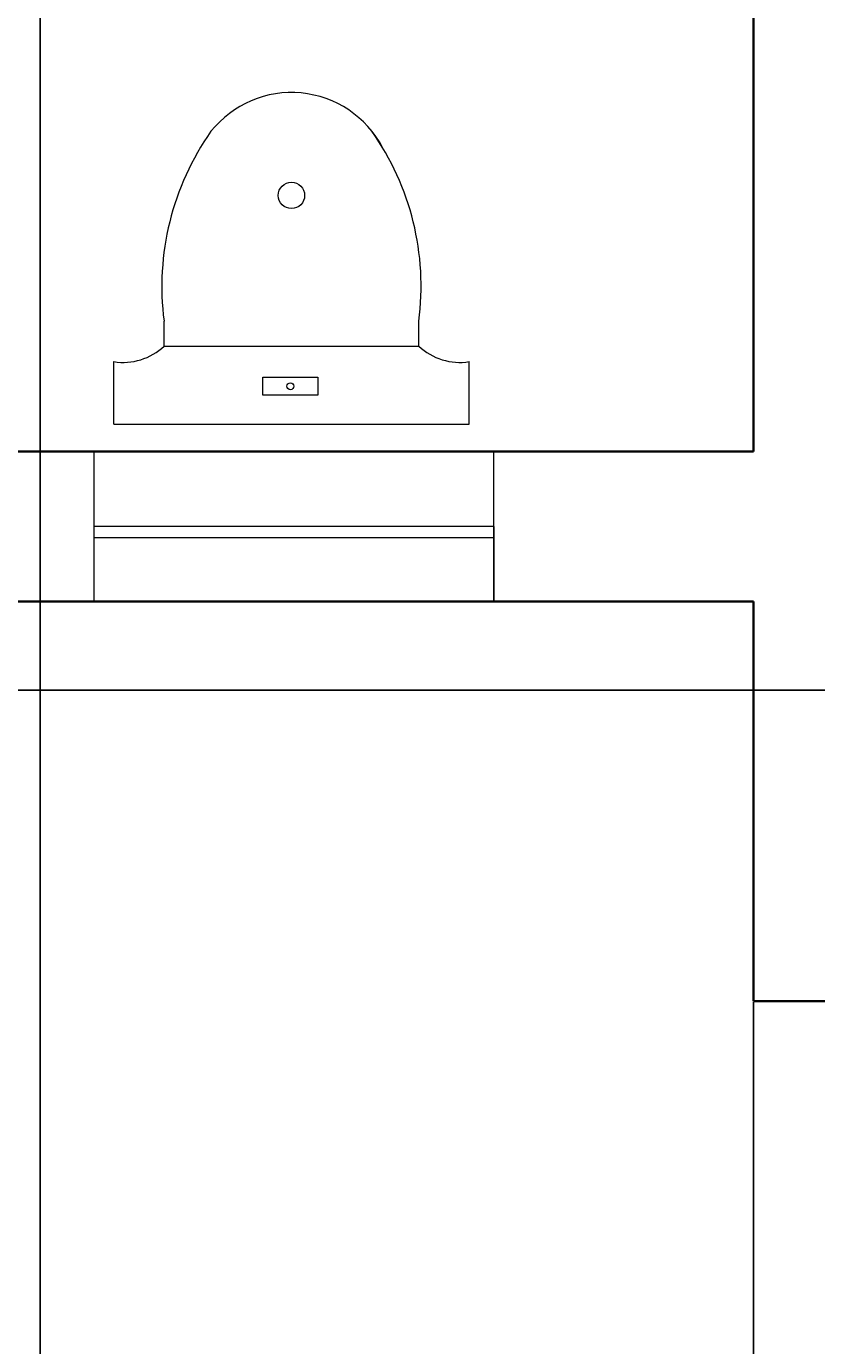
# Model space of a CAD drawing. Units: inches. Extents: x -61 to 1599, y -1316 to 257.
# Tile 79 of 204: x 276 to 323, y -486 to -407. Entities that reach past the tile are written whole.
import ezdxf

# ---------------------------------------------------------------- set-up
doc = ezdxf.new("R2010")
doc.units = ezdxf.units.IN
doc.header["$MEASUREMENT"] = 0
for name, color, linetype, lineweight in [('A-ANNO-DIMS', 2, 'Continuous', 18), ('A-FLOR-FIXT', 8, 'Continuous', 18), ('WALLS', 4, 'Continuous', 35), ('WINDOWS', 220, 'Continuous', 18)]:
    doc.layers.add(name, color=color, linetype=linetype, lineweight=lineweight)
doc.styles.get("Standard").update_dxf_attribs({"font": 'arial.ttf'})
doc.dimstyles.get("Standard").update_dxf_attribs({"dimtxt": 0.18, "dimasz": 0.18, "dimexe": 0.18, "dimexo": 0.0625, "dimgap": 0.09, "dimtad": 0, "dimtih": 1, "dimtoh": 1, "dimdec": 0, "dimzin": 0, "dimdsep": 46, "dimlunit": 3, "dimtxsty": 'Standard', "dimcen": 0.09, "dimadec": 0, "dimazin": 0, "dimtfac": 1, "dimtdec": 0, "dimtofl": 0, "dimtmove": 0, "dimatfit": 3, "dimfxl": 1, "dimtolj": 1, "dimtzin": 0, "dimarcsym": 0})

# ---------------------------------------------------------------- blocks, each defined once
blk = doc.blocks.new('WIN-24IN')
for p, q in [((0, 4.5), (0, 9)), ((0, 9), (0, 0)), ((24, 9), (24, 0)), ((0, 5.192), (24, 5.192)), ((0, 4.5), (24, 4.5))]:
    blk.add_line(p, q)
blk = doc.blocks.new('WC-FLOOR-MOUNT')
for p, q in [((3.018, 4.686), (3.018, 6.173)), ((18.314, 4.686), (18.314, 6.173)), ((3.018, 4.686), (18.314, 4.686)), ((0, 0), (0, 3.747)), ((21.331, 0), (21.331, 3.747)), ((0, 0), (21.331, 0))]:
    blk.add_line(p, q)
blk.add_lwpolyline([(12.243, 1.734), (8.955, 1.734), (8.955, 2.812), (12.243, 2.812)], close=True)
for centre, radius in [((10.666, 13.729), 0.792), ((10.599, 2.273), 0.208)]:
    blk.add_circle(centre, radius)
for centre, radius, start, end in [((10.666, 13.729), 6.176, 27.68441, 141.46969), ((19.051, 8.262), 16.169, 144.82396, 187.42318), ((2.281, 8.262), 16.169, 352.57682, 35.17604), ((0.565, 7.253), 3.551, 260.8586, 313.6993), ((20.767, 7.253), 3.551, 226.3007, 279.1414)]:
    blk.add_arc(centre, radius, start, end)
blk = doc.blocks.new('*D687')
at = {"layer": 'A-ANNO-DIMS', "color": 0, "lineweight": -2, "transparency": 16777216}
for p, q in [((289.418, 181.677), (-61.077, 181.677)), ((-60.897, 181.497), (-60.897, -528.952)), ((-60.897, -1239.765), (-60.897, -529.316)), ((319.64, -1239.945), (-61.077, -1239.945))]:
    blk.add_line(p, q, dxfattribs=at)
at = {"layer": 'A-ANNO-DIMS', "color": 0, "transparency": 16777216}
for points in [[(-60.927, 181.497), (-60.867, 181.497), (-60.897, 181.677)], [(-60.927, -1239.765), (-60.867, -1239.765), (-60.897, -1239.945)]]:
    blk.add_solid(points, dxfattribs=at)
at = {"layer": 'DEFPOINTS', "color": 0, "transparency": 16777216}
for p in [(289.481, 181.677), (-60.897, -1239.945), (319.703, -1239.945)]:
    blk.add_point(p, dxfattribs=at)
at = {"layer": 'A-ANNO-DIMS', "color": 0, "transparency": 16777216, "insert": (-60.897, -529.134), "char_height": 0.18, "attachment_point": 5}
blk.add_mtext('\\A1;1421.6', dxfattribs=at)
blk = doc.blocks.new('*D699')
at = {"layer": 'A-ANNO-DIMS', "color": 0, "lineweight": -2, "transparency": 16777216}
for p, q in [((835.64, -167.169), (-61.077, -167.169)), ((-60.897, -167.349), (-60.897, -306.726)), ((-60.897, -446.466), (-60.897, -307.09)), ((841.64, -446.646), (-61.077, -446.646))]:
    blk.add_line(p, q, dxfattribs=at)
at = {"layer": 'A-ANNO-DIMS', "color": 0, "transparency": 16777216}
for points in [[(-60.927, -167.349), (-60.867, -167.349), (-60.897, -167.169)], [(-60.927, -446.466), (-60.867, -446.466), (-60.897, -446.646)]]:
    blk.add_solid(points, dxfattribs=at)
at = {"layer": 'DEFPOINTS', "color": 0, "transparency": 16777216}
for p in [(835.703, -167.169), (-60.897, -446.646), (841.703, -446.646)]:
    blk.add_point(p, dxfattribs=at)
at = {"layer": 'A-ANNO-DIMS', "color": 0, "transparency": 16777216, "insert": (-60.897, -306.908), "char_height": 0.18, "attachment_point": 5}
blk.add_mtext('\\A1;279.5', dxfattribs=at)
blk = doc.blocks.new('*D702')
at = {"layer": 'A-ANNO-DIMS', "color": 0, "lineweight": -2, "transparency": 16777216}
for p, q in [((276.882, -616.882), (276.882, 257.457)), ((348.32, -616.882), (348.32, 257.457)), ((277.062, 257.277), (312.209, 257.277)), ((348.14, 257.277), (312.994, 257.277))]:
    blk.add_line(p, q, dxfattribs=at)
at = {"layer": 'A-ANNO-DIMS', "color": 0, "transparency": 16777216}
for points in [[(277.062, 257.307), (277.062, 257.247), (276.882, 257.277)], [(348.14, 257.307), (348.14, 257.247), (348.32, 257.277)]]:
    blk.add_solid(points, dxfattribs=at)
at = {"layer": 'DEFPOINTS', "color": 0, "transparency": 16777216}
for p in [(348.32, 257.277), (276.882, -616.945), (348.32, -616.945)]:
    blk.add_point(p, dxfattribs=at)
at = {"layer": 'A-ANNO-DIMS', "color": 0, "transparency": 16777216, "insert": (312.601, 257.277), "char_height": 0.18, "attachment_point": 5}
blk.add_mtext('\\A1;71.44', dxfattribs=at)
blk = doc.blocks.new('*D710')
at = {"layer": 'A-ANNO-DIMS', "color": 0, "lineweight": -2, "transparency": 16777216}
for p, q in [((319.703, -465.385), (319.703, -1315.725)), ((403.703, -465.385), (403.703, -1315.725)), ((319.883, -1315.545), (361.484, -1315.545)), ((403.523, -1315.545), (361.921, -1315.545))]:
    blk.add_line(p, q, dxfattribs=at)
at = {"layer": 'A-ANNO-DIMS', "color": 0, "transparency": 16777216}
for points in [[(319.883, -1315.515), (319.883, -1315.575), (319.703, -1315.545)], [(403.523, -1315.515), (403.523, -1315.575), (403.703, -1315.545)]]:
    blk.add_solid(points, dxfattribs=at)
at = {"layer": 'DEFPOINTS', "color": 0, "transparency": 16777216}
for p in [(319.703, -465.323), (403.703, -465.323), (403.703, -1315.545)]:
    blk.add_point(p, dxfattribs=at)
at = {"layer": 'A-ANNO-DIMS', "color": 0, "transparency": 16777216, "insert": (361.703, -1315.545), "char_height": 0.18, "attachment_point": 5}
blk.add_mtext('\\A1;84', dxfattribs=at)

msp = doc.modelspace()

# ---------------------------------------------------------------- linework, layer by layer
at = {"layer": 'WALLS'}
for p, q in [((319.7028, -400.2167), (319.7028, -432.3229)), ((265.7028, -432.3229), (319.7028, -432.3229)), ((237.7028, -441.3229), (319.7028, -441.3229)), ((319.7028, -441.3229), (319.7028, -465.3229)), ((403.7028, -465.3229), (319.7028, -465.3229))]:
    msp.add_line(p, q, dxfattribs=at)

# ---------------------------------------------------------------- block references
at = {"layer": 'A-FLOR-FIXT'}
msp.add_blockref('WC-FLOOR-MOUNT', (281.2982, -430.6752), dxfattribs=at)
at = {"layer": 'WINDOWS', "rotation": 180}
msp.add_blockref('WIN-24IN', (304.1139, -432.3228), dxfattribs=at)

# ---------------------------------------------------------------- dimensions: what is measured, and where the dimension line sits
at = {"layer": 'A-ANNO-DIMS'}
for base, p1, p2, override, picture, middle in [((348.3201, 257.2771), (276.8825, -616.9446), (348.3201, -616.9446), {"dimdec": 2, "dimlfac": 1, "dimrnd": 0, "dimzin": 0, "dimdsep": 46, "dimlunit": 2}, '*D702', (312.6013, 257.2771)), ((403.7028, -1315.5446), (319.7028, -465.3229), (403.7028, -465.3229), {"dimdec": 0, "dimlfac": 1, "dimrnd": 0, "dimzin": 0, "dimdsep": 46, "dimlunit": 2}, '*D710', (361.7028, -1315.5446))]:
    dim = msp.add_linear_dim(base=base, p1=p1, p2=p2, dimstyle='Standard', override=override, dxfattribs=at)
    dim.commit()
    dim.dimension.update_dxf_attribs({"geometry": picture, "text_midpoint": middle})
for base, p1, p2, picture, middle in [((-60.8972, -1239.9446), (289.4807, 181.6771), (319.7028, -1239.9446), '*D687', (-60.8972, -529.1337)), ((-60.8972, -446.6462), (835.7028, -167.169), (841.7028, -446.6462), '*D699', (-60.8972, -306.9076))]:
    dim = msp.add_linear_dim(base=base, p1=p1, p2=p2, angle=90, dimstyle='Standard', override={"dimdec": 1, "dimlfac": 1, "dimrnd": 0, "dimzin": 0, "dimdsep": 46, "dimlunit": 2}, dxfattribs=at)
    dim.commit()
    dim.dimension.update_dxf_attribs({"geometry": picture, "text_midpoint": middle})

doc.saveas('drawing.dxf')
